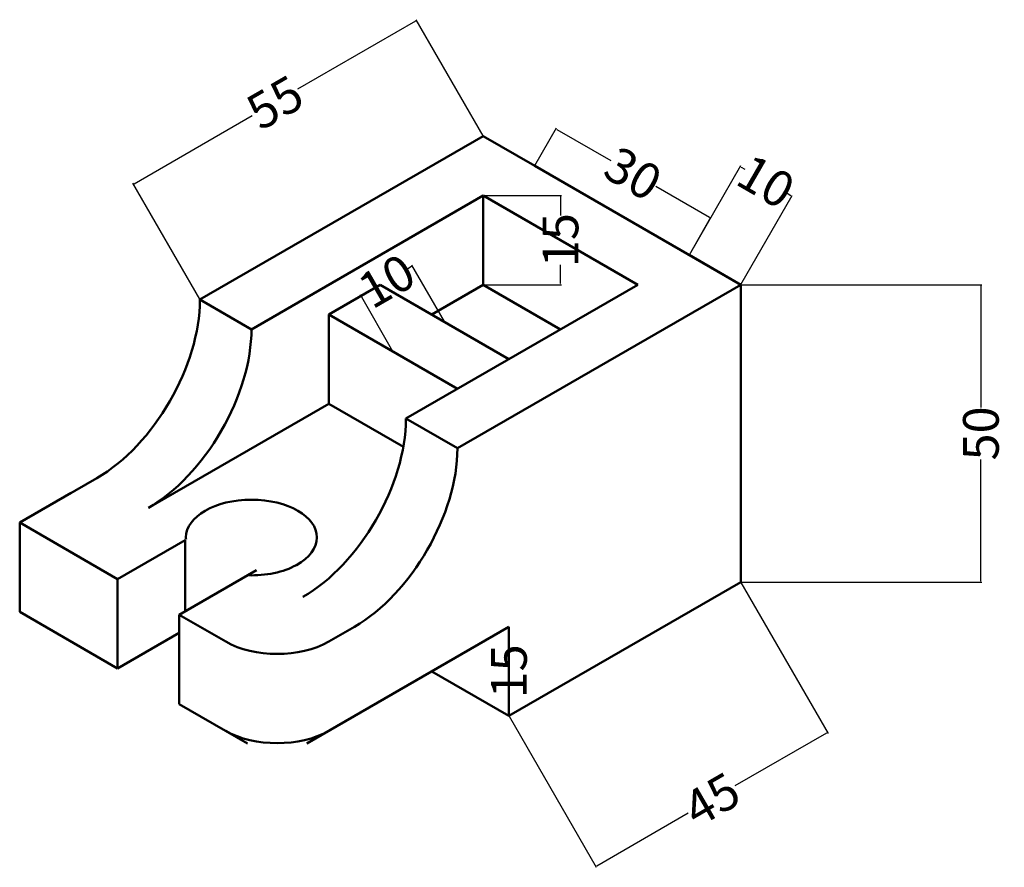
# Model space of a CAD drawing. Units: millimetres. Extents: x -29 to 137, y 6 to 149.
import ezdxf

# ---------------------------------------------------------------- set-up
doc = ezdxf.new("R2010")
doc.units = ezdxf.units.MM
doc.header["$MEASUREMENT"] = 0
doc.layers.add('M-DIMS', color=2, linetype='Continuous', lineweight=25)
doc.layers.add('M-OUTL', color=7, linetype='Continuous', lineweight=50)
doc.styles.get("Standard").update_dxf_attribs({"font": 'arial.ttf'})
doc.dimstyles.get("Standard").update_dxf_attribs({"dimtxt": 6, "dimasz": 0.18, "dimexe": 0.18, "dimexo": 0.0625, "dimgap": 0.09, "dimtad": 0, "dimtoh": 1, "dimdec": 0, "dimzin": 0, "dimdsep": 46, "dimtxsty": 'Standard', "dimcen": 0.09, "dimadec": 0, "dimazin": 0, "dimtfac": 1, "dimtdec": 0, "dimtofl": 0, "dimtmove": 0, "dimatfit": 3, "dimfxl": 1, "dimtolj": 1, "dimtzin": 0, "dimarcsym": 0})

# ---------------------------------------------------------------- blocks, each defined once
blk = doc.blocks.new('*D1')
at = {"layer": 'Defpoints', "color": 0, "transparency": 16777216}
for p in [(53.53, 46.52), (53.53, 31.52), (53.53, 31.52)]:
    blk.add_point(p, dxfattribs=at)
at = {"layer": 'M-DIMS', "color": 0, "lineweight": -2, "transparency": 16777216}
for p, q in [((53.47, 46.52), (53.35, 46.52)), ((53.53, 46.34), (53.53, 43.15)), ((53.53, 31.7), (53.53, 34.89)), ((53.47, 31.52), (53.35, 31.52))]:
    blk.add_line(p, q, dxfattribs=at)
at = {"layer": 'M-DIMS', "color": 0, "transparency": 16777216}
for points in [[(53.5, 46.34), (53.56, 46.34), (53.53, 46.52)], [(53.5, 31.7), (53.56, 31.7), (53.53, 31.52)]]:
    blk.add_solid(points, dxfattribs=at)
at = {"layer": 'M-DIMS', "color": 0, "transparency": 16777216, "insert": (53.53, 39.02), "char_height": 6, "attachment_point": 5, "rotation": 90}
blk.add_mtext('\\A1;15', dxfattribs=at)
blk = doc.blocks.new('*D2')
at = {"layer": 'Defpoints', "color": 0, "transparency": 16777216}
for p in [(57.86, 124.02), (87.41, 115.21), (83.84, 109.02)]:
    blk.add_point(p, dxfattribs=at)
at = {"layer": 'M-DIMS', "color": 0, "lineweight": -2, "transparency": 16777216}
for p, q in [((57.89, 124.07), (61.52, 130.37)), ((61.59, 130.12), (70.64, 124.9)), ((87.26, 115.3), (78.21, 120.52)), ((83.87, 109.07), (87.5, 115.37))]:
    blk.add_line(p, q, dxfattribs=at)
at = {"layer": 'M-DIMS', "color": 0, "transparency": 16777216}
for points in [[(61.61, 130.15), (61.58, 130.09), (61.43, 130.21)], [(87.27, 115.33), (87.24, 115.27), (87.41, 115.21)]]:
    blk.add_solid(points, dxfattribs=at)
at = {"layer": 'M-DIMS', "color": 0, "transparency": 16777216, "insert": (74.42, 122.71), "char_height": 6, "attachment_point": 5, "rotation": 330}
blk.add_mtext('\\A1;30', dxfattribs=at)
blk = doc.blocks.new('*D3')
at = {"layer": 'Defpoints', "color": 0, "transparency": 16777216}
for p in [(92.5, 54.02), (53.53, 31.52), (107.1, 28.73)]:
    blk.add_point(p, dxfattribs=at)
at = {"layer": 'M-DIMS', "color": 0, "lineweight": -2, "transparency": 16777216}
for p, q in [((92.53, 53.97), (107.19, 28.58)), ((53.56, 31.47), (68.22, 6.08)), ((106.95, 28.64), (91.54, 19.75)), ((68.29, 6.32), (83.69, 15.22))]:
    blk.add_line(p, q, dxfattribs=at)
at = {"layer": 'M-DIMS', "color": 0, "transparency": 16777216}
for points in [[(106.93, 28.67), (106.96, 28.62), (107.1, 28.73)], [(68.27, 6.35), (68.3, 6.3), (68.13, 6.23)]]:
    blk.add_solid(points, dxfattribs=at)
at = {"layer": 'M-DIMS', "color": 0, "transparency": 16777216, "insert": (87.62, 17.48), "char_height": 6, "attachment_point": 5, "rotation": 30}
blk.add_mtext('\\A1;45', dxfattribs=at)
blk = doc.blocks.new('*D4')
at = {"layer": 'Defpoints', "color": 0, "transparency": 16777216}
for p in [(92.5, 104.02), (92.5, 54.02), (132.89, 54.02)]:
    blk.add_point(p, dxfattribs=at)
at = {"layer": 'M-DIMS', "color": 0, "lineweight": -2, "transparency": 16777216}
for p, q in [((92.56, 104.02), (133.07, 104.02)), ((132.89, 103.84), (132.89, 83.4)), ((132.89, 54.2), (132.89, 74.64)), ((92.56, 54.02), (133.07, 54.02))]:
    blk.add_line(p, q, dxfattribs=at)
at = {"layer": 'M-DIMS', "color": 0, "transparency": 16777216}
for points in [[(132.86, 103.84), (132.92, 103.84), (132.89, 104.02)], [(132.86, 54.2), (132.92, 54.2), (132.89, 54.02)]]:
    blk.add_solid(points, dxfattribs=at)
at = {"layer": 'M-DIMS', "color": 0, "transparency": 16777216, "insert": (132.89, 79.02), "char_height": 6, "attachment_point": 5, "rotation": 90}
blk.add_mtext('\\A1;50', dxfattribs=at)
blk = doc.blocks.new('*D5')
at = {"layer": 'Defpoints', "color": 0, "transparency": 16777216}
for p in [(49.2, 129.02), (-9.63, 120.92), (1.57, 101.52)]:
    blk.add_point(p, dxfattribs=at)
at = {"layer": 'M-DIMS', "color": 0, "lineweight": -2, "transparency": 16777216}
for p, q in [((37.84, 148.33), (18, 136.88)), ((49.17, 129.07), (37.91, 148.58)), ((-9.48, 121.01), (10.36, 132.47)), ((1.54, 101.57), (-9.72, 121.08))]:
    blk.add_line(p, q, dxfattribs=at)
at = {"layer": 'M-DIMS', "color": 0, "transparency": 16777216}
for points in [[(37.83, 148.36), (37.86, 148.31), (38, 148.42)], [(-9.49, 121.04), (-9.46, 120.99), (-9.63, 120.92)]]:
    blk.add_solid(points, dxfattribs=at)
at = {"layer": 'M-DIMS', "color": 0, "transparency": 16777216, "insert": (14.18, 134.67), "char_height": 6, "attachment_point": 5, "rotation": 30}
blk.add_mtext('\\A1;55', dxfattribs=at)
blk = doc.blocks.new('*D6')
at = {"layer": 'Defpoints', "color": 0, "transparency": 16777216}
for p in [(28.63, 102.15), (42.7, 97.77), (34.04, 92.77)]:
    blk.add_point(p, dxfattribs=at)
at = {"layer": 'M-DIMS', "color": 0, "lineweight": -2, "transparency": 16777216}
for p, q in [((37.14, 107.06), (36.51, 106.69)), ((42.67, 97.82), (37.2, 107.3)), ((34.01, 92.82), (28.54, 102.3)), ((28.79, 102.24), (29.42, 102.6))]:
    blk.add_line(p, q, dxfattribs=at)
at = {"layer": 'M-DIMS', "color": 0, "transparency": 16777216}
for points in [[(37.12, 107.08), (37.15, 107.03), (37.29, 107.15)], [(28.77, 102.26), (28.8, 102.21), (28.63, 102.15)]]:
    blk.add_solid(points, dxfattribs=at)
at = {"layer": 'M-DIMS', "color": 0, "transparency": 16777216, "insert": (32.96, 104.65), "char_height": 6, "attachment_point": 5, "rotation": 30}
blk.add_mtext('\\A1;10', dxfattribs=at)
blk = doc.blocks.new('*D7')
at = {"layer": 'Defpoints', "color": 0, "transparency": 16777216}
for p in [(101.09, 118.89), (83.84, 109.02), (92.5, 104.02)]:
    blk.add_point(p, dxfattribs=at)
at = {"layer": 'M-DIMS', "color": 0, "lineweight": -2, "transparency": 16777216}
for p, q in [((83.87, 109.07), (92.51, 124.04)), ((92.58, 123.8), (93.21, 123.44)), ((100.93, 118.98), (100.3, 119.34)), ((92.53, 104.07), (101.18, 119.04))]:
    blk.add_line(p, q, dxfattribs=at)
at = {"layer": 'M-DIMS', "color": 0, "transparency": 16777216}
for points in [[(92.6, 123.82), (92.57, 123.77), (92.42, 123.89)], [(100.94, 119), (100.91, 118.95), (101.09, 118.89)]]:
    blk.add_solid(points, dxfattribs=at)
at = {"layer": 'M-DIMS', "color": 0, "transparency": 16777216, "insert": (96.75, 121.39), "char_height": 6, "attachment_point": 5, "rotation": 330}
blk.add_mtext('\\A1;10', dxfattribs=at)
blk = doc.blocks.new('*D8')
at = {"layer": 'Defpoints', "color": 0, "transparency": 16777216}
for p in [(49.2, 119.02), (49.2, 104.02), (62.19, 104.02)]:
    blk.add_point(p, dxfattribs=at)
at = {"layer": 'M-DIMS', "color": 0, "lineweight": -2, "transparency": 16777216}
for p, q in [((49.26, 119.02), (62.37, 119.02)), ((62.19, 118.84), (62.19, 115.65)), ((62.19, 104.2), (62.19, 107.39)), ((49.26, 104.02), (62.37, 104.02))]:
    blk.add_line(p, q, dxfattribs=at)
at = {"layer": 'M-DIMS', "color": 0, "transparency": 16777216}
for points in [[(62.16, 118.84), (62.22, 118.84), (62.19, 119.02)], [(62.16, 104.2), (62.22, 104.2), (62.19, 104.02)]]:
    blk.add_solid(points, dxfattribs=at)
at = {"layer": 'M-DIMS', "color": 0, "transparency": 16777216, "insert": (62.19, 111.52), "char_height": 6, "attachment_point": 5, "rotation": 90}
blk.add_mtext('\\A1;15', dxfattribs=at)

msp = doc.modelspace()

# ---------------------------------------------------------------- linework, layer by layer
at = {"layer": 'M-OUTL'}
for p, q in [((49.2, 129.02), (1.57, 101.52)), ((57.86, 124.02), (49.2, 129.02)), ((92.5, 104.02), (57.86, 124.02)), ((10.23, 96.52), (49.2, 119.02)), ((75.18, 104.02), (49.2, 119.02)), ((49.2, 119.02), (49.2, 104.02)), ((92.5, 104.02), (83.84, 109.02)), ((27.72, 106.62), (27.69, 106.64)), ((23.22, 99.02), (31.88, 104.02)), ((53.53, 91.52), (31.88, 104.02)), ((36.21, 81.52), (75.18, 104.02)), ((49.2, 104.02), (40.54, 99.02)), ((92.5, 104.02), (44.87, 76.52)), ((49.2, 104.02), (62.19, 96.52)), ((92.5, 54.02), (92.5, 104.02)), ((10.23, 96.52), (1.57, 101.52)), ((23.22, 84.02), (23.22, 99.02)), ((23.22, 99.02), (44.87, 86.52)), ((-7.09, 66.52), (23.22, 84.02)), ((23.22, 84.02), (35.77, 76.78)), ((44.87, 76.52), (36.21, 81.52)), ((-15.75, 71.52), (-28.74, 64.02)), ((-28.74, 64.02), (-20.08, 69.02)), ((-28.74, 64.02), (-22.25, 67.77)), ((-22.25, 67.77), (-22.25, 67.77)), ((-28.74, 64.02), (-12.29, 54.52)), ((-28.74, 64.02), (-28.74, 49.02)), ((-28.74, 64.02), (-28.74, 54.02)), ((-0.91, 61.09), (-12.29, 54.52)), ((-0.91, 61.09), (-0.91, 49.09)), ((11.09, 56.02), (-1.9, 48.52)), ((-12.29, 39.52), (-12.29, 54.52)), ((53.53, 31.52), (92.5, 54.02)), ((-28.74, 49.02), (-12.29, 39.52)), ((-1.9, 33.52), (-1.9, 48.52)), ((-1.9, 48.52), (5.9, 44.02)), ((53.53, 46.52), (19.56, 26.91)), ((23.22, 44.02), (27.55, 46.52)), ((53.53, 31.52), (53.53, 46.52)), ((-12.29, 39.52), (-1.9, 45.52)), ((53.53, 31.52), (40.54, 39.02)), ((9.56, 26.91), (-1.9, 33.52))]:
    msp.add_line(p, q, dxfattribs=at)
msp.add_lwpolyline([(44.87, 76.52), (92.5, 104.02)], dxfattribs=at)
for centre, major_axis, start_param, end_param in [((-15.75, 91.52), (-12.25, -21.21), 0.785398, 2.356194), ((-7.09, 86.52), (-12.25, -21.21), 7.068583, 8.63938), ((18.89, 71.52), (-12.25, -21.21), 0.785398, 2.356194), ((27.55, 66.52), (-12.25, -21.21), 0.785398, 2.356194), ((10.23, 61.52), (-11.02, 0), 3.141593, 6.283185), ((10.23, 61.52), (-11.02, 0), 0, 0.055671), ((10.23, 61.52), (-11.02, 0), 1.515126, 3.141593), ((14.56, 49.02), (12.25, 0), 3.926991, 5.497787), ((14.56, 34.02), (12.25, 0), 3.926991, 5.497787)]:
    msp.add_ellipse(centre, major_axis=major_axis, ratio=0.57735, start_param=start_param, end_param=end_param, dxfattribs=at)

# ---------------------------------------------------------------- dimensions: what is measured, and where the dimension line sits
at = {"layer": 'M-DIMS'}
for p1, p2, distance, picture, middle in [((49.2, 129.02), (1.57, 101.52), -22.4, '*D5', (14.18, 134.67)), ((57.86, 124.02), (83.84, 109.02), 7.15, '*D2', (74.42, 122.71)), ((83.84, 109.02), (92.5, 104.02), 17.17, '*D7', (96.75, 121.39)), ((49.2, 119.02), (49.2, 104.02), 12.99, '*D8', (62.19, 111.52)), ((42.7, 97.77), (34.04, 92.77), -10.83, '*D6', (32.96, 104.65)), ((92.5, 104.02), (92.5, 54.02), 40.39, '*D4', (132.89, 79.02)), ((53.53, 31.52), (92.5, 54.02), -29.2, '*D3', (87.62, 17.48)), ((53.53, 46.52), (53.53, 31.52), 0, '*D1', (53.53, 39.02))]:
    dim = msp.add_aligned_dim(p1=p1, p2=p2, distance=distance, dimstyle='Standard', override={"dimclrd": 0, "dimclre": 0, "dimclrt": 0}, dxfattribs=at)
    dim.commit()
    dim.dimension.update_dxf_attribs({"geometry": picture, "text_midpoint": middle})

doc.saveas('drawing.dxf')
